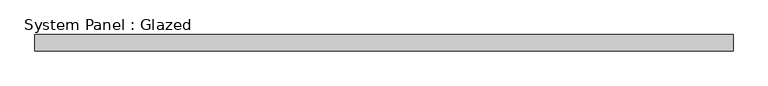
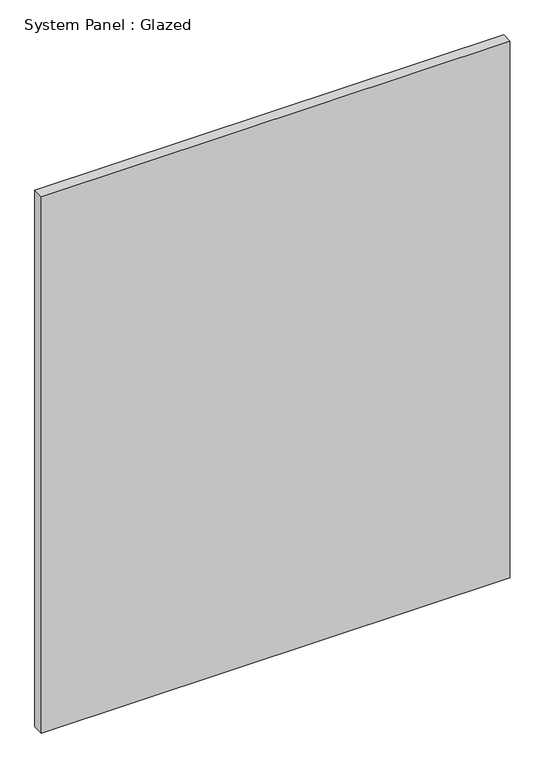
"""IFC4 building model written with IfcOpenShell, lengths in millimetres: plate geometry, System Panel : Glazed."""

from ifc_helpers import new_model, si_unit, origin, origin_with_axes, place, context, project, spatial, polyline, outline, extrude, source, transform, mapped, element, save


def system_panel_glazed_e6353eef(model_context):
    return source(origin(), model_context, "Body", "SweptSolid", [
        extrude(outline(polyline([(546.1, 19.05), (-546.1, 19.05), (-546.1, 44.45), (546.1, 44.45), (546.1, 19.05)])), origin_with_axes(), (0.0, 0.0, 1.0), 1320.8),
    ])


if __name__ == "__main__":
    model = new_model("IFC4")
    model_context = context("Model", 3, world=origin())
    ifc_project = project(units=[si_unit("LENGTHUNIT", "METRE", prefix="MILLI")], contexts=[model_context])
    site = spatial("IfcSite", under=ifc_project)
    building = spatial("IfcBuilding", under=site)
    placement = place(None, origin())
    system_panel_glazed_shape = system_panel_glazed_e6353eef(model_context)
    element("IfcPlate", 1, ObjectType="System Panel : Glazed", at=placement, inside=building, context=model_context, shape_type="MappedRepresentation", body=[
        mapped(system_panel_glazed_shape, transform((0.0, 0.0, 0.0), x_axis=(1.0, 0.0, 0.0), y_axis=(0.0, 1.0, 0.0), z_axis=(0.0, 0.0, 1.0))),
    ])
    save(model, "model.ifc")

# Revit data of these elements
# Type "System Panel : Glazed"
#   Construction Type Id = "GSP4R"
#   Analytic Construction = "1/8 in Pilkington single glazing"
#   Visual Light Transmittance = 0.9
#   Solar Heat Gain Coefficient = 0.86
#   Heat Transfer Coefficient (U) = 1.18115 BTU/(h·ft²·°F)
#   Define Thermal Properties by = 1
# Element 1 (IfcPlate, "System Panel : Glazed")
#   Materials on its faces: "Glass"
# Materials
#   "Glass": class "Glass", colour RGB 0 128 192, transparency 0.75, Description = "Soda Lime Glass", Cost = 0
